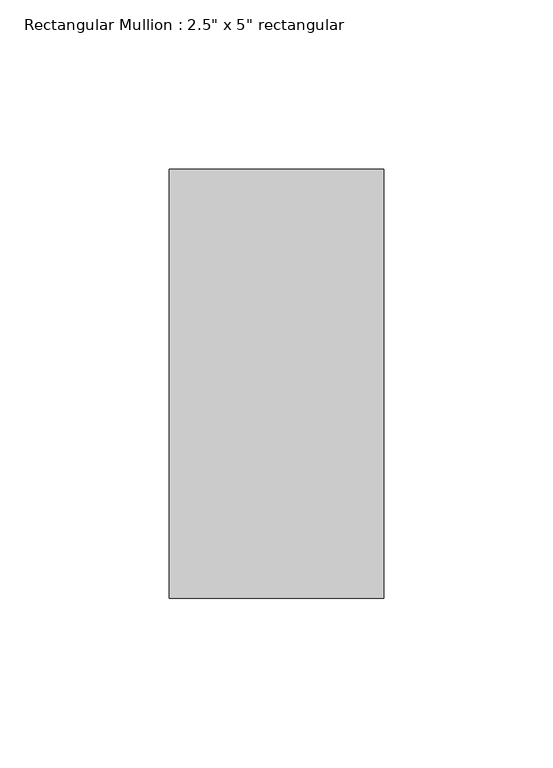
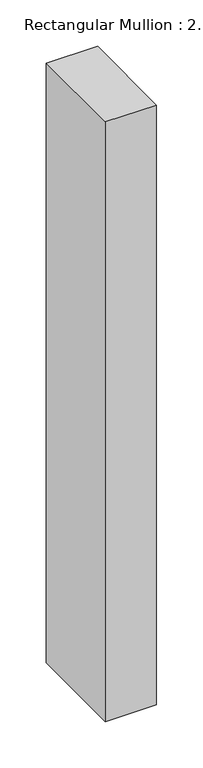
"""IFC4 building model written with IfcOpenShell, lengths in millimetres: member geometry."""

from ifc_helpers import new_model, si_unit, frame, origin, place, context, project, spatial, polyline, outline, extrude, source, transform, mapped, element, save


def member_8b7748c8(model_context):
    return source(origin(), model_context, "Body", "SweptSolid", [
        extrude(outline(polyline([(31.75, 63.5), (31.75, -63.5), (-31.75, -63.5), (-31.75, 63.5), (31.75, 63.5)])), frame((0.0, 0.0, -788.2127727), z_axis=(0.0, 0.0, 1.0), x_axis=(1.0, 0.0, 0.0)), (0.0, 0.0, 1.0), 788.2127727),
    ])


if __name__ == "__main__":
    model = new_model("IFC4")
    model_context = context("Model", 3, world=origin())
    ifc_project = project(units=[si_unit("LENGTHUNIT", "METRE", prefix="MILLI")], contexts=[model_context])
    site = spatial("IfcSite", under=ifc_project)
    building = spatial("IfcBuilding", under=site)
    placement = place(None, origin())
    member_shape = member_8b7748c8(model_context)
    element("IfcMember", 1, ObjectType="Rectangular Mullion : 2.5\" x 5\" rectangular", at=placement, inside=building, context=model_context, shape_type="MappedRepresentation", body=[
        mapped(member_shape, transform((0.0, 0.0, 0.0), x_axis=(1.0, 0.0, 0.0), y_axis=(0.0, 1.0, 0.0), z_axis=(0.0, 0.0, 1.0))),
    ])
    save(model, "model.ifc")

# Revit data of these elements
# Type "Rectangular Mullion : 2.5\" x 5\" rectangular"
#   built-in parameter 1007304 = 0.416667 (stored number, unit not read)
#   built-in parameter 1007301 = 0.104167 (stored number, unit not read)
#   built-in parameter 1007300 = 0.104167 (stored number, unit not read)
# Element 1 (IfcMember, "Rectangular Mullion : 2.5\" x 5\" rectangular")
#   Materials on its faces: "Aluminum"
# Materials
#   "Aluminum": class "Metal", colour RGB 247 247 247, transparency 0, Description = "Aluminum 6061", Cost = 0
